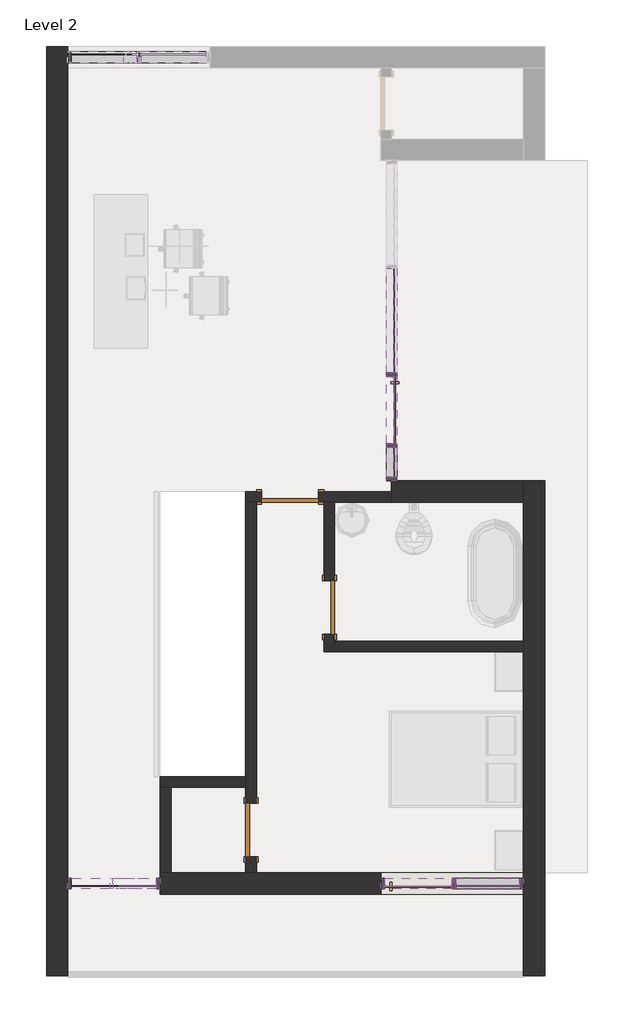
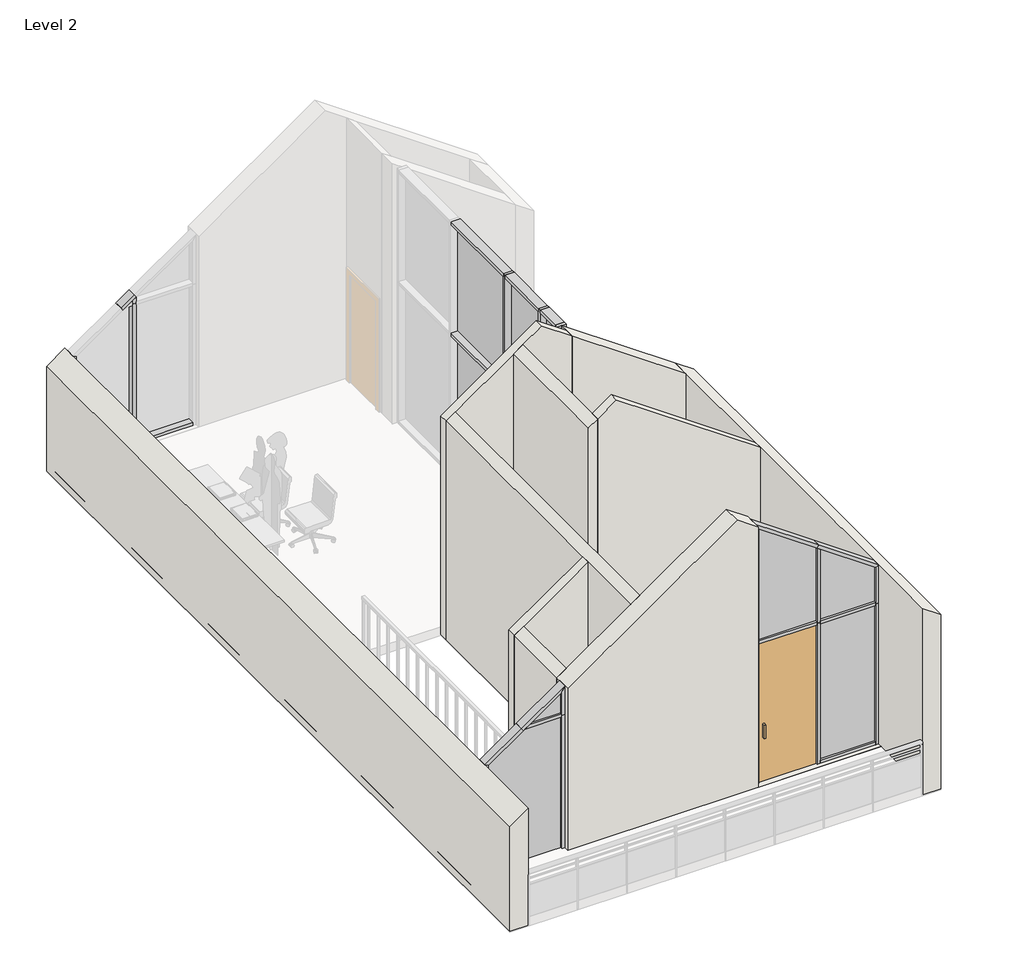
# One storey, part 1 of 2: 37 members, 10 plates, 10 walls, 5 doors.
"""IFC4 building model written with IfcOpenShell, lengths in millimetres."""

from ifc_helpers import new_model, si_unit, frame, origin, place, context, project, spatial, polyline, outline, extrude, faceted_brep, transform, mapped, element, save
from components import m_door_curtain_wall_single_glass_m_door_curtain_wall_single_b00c2793, m_door_curtain_wall_single_glass_m_door_curtain_wall_single_a386b0a2, m_door_single_flush_panel_double_acting_750_x_2000mm_e3d998e5, m_door_single_panel_750_x_2000mm_5cf0dcc2, m_door_single_panel_800_x_2100mm_d01656e8, rectangular_mullion_50_x_150mm_a91aaa2b, rectangular_mullion_50_x_150mm_6588f46c, rectangular_mullion_50_x_150mm_89c22e8d, rectangular_mullion_50_x_150mm_2615a836, rectangular_mullion_50_x_150mm_129a33a7, rectangular_mullion_50_x_150mm_c59a77fc, rectangular_mullion_50_x_150mm_4a18de0c, rectangular_mullion_50_x_150mm_a16d5dba, rectangular_mullion_50_x_150mm_59b4522d, rectangular_mullion_50_x_150mm_a5bab1e1, rectangular_mullion_50_x_150mm_e6be0bb7, rectangular_mullion_50_x_150mm_987ee5f5, rectangular_mullion_50_x_150mm_e09f09b0, rectangular_mullion_50_x_150mm_fd5e96fe, rectangular_mullion_50_x_150mm_9159db86, rectangular_mullion_50_x_150mm_405b5ff6, rectangular_mullion_50_x_150mm_a3343b62, rectangular_mullion_50_x_150mm_bd832bbd, rectangular_mullion_50_x_150mm_0164b494, rectangular_mullion_50_x_150mm_17c629a1, rectangular_mullion_50_x_150mm_35d6a770, rectangular_mullion_50_x_150mm_dd699d0b, rectangular_mullion_50_x_150mm_0e9b4e8c, rectangular_mullion_50_x_150mm_bef26404, rectangular_mullion_50_x_150mm_3ddb3363, rectangular_mullion_50_x_150mm_71cd5d06, rectangular_mullion_50_x_150mm_6afb4452, rectangular_mullion_50_x_150mm_b2f97b5b, system_panel_glazed_5205d833, system_panel_glazed_35c1503a, system_panel_glazed_def3cda3, system_panel_glazed_393e2e5d, system_panel_glazed_fc828323, system_panel_glazed_9e355314, system_panel_glazed_94ea2f12, system_panel_glazed_9142b3e3, system_panel_glazed_bc7b3e81, system_panel_glazed_03cdf4a0

model = new_model("IFC4")

# Units and contexts
model_context = context("Model", 3, world=origin())
ifc_project = project(units=[si_unit("LENGTHUNIT", "METRE", prefix="MILLI")], contexts=[model_context])

# Site, building, storey
site = spatial("IfcSite", under=ifc_project)
building = spatial("IfcBuilding", under=site)
storey = spatial("IfcBuildingStorey", under=building, Name="Level 2", Elevation=3200.0)

# Doors
placement = place(None, origin())
m_door_curtain_wall_single_glass_m_door_curtain_wall_single_shape = m_door_curtain_wall_single_glass_m_door_curtain_wall_single_b00c2793(model_context)
element("IfcDoor", 1, ObjectType="M_Door-Curtain-Wall-Single-Glass : M_Door-Curtain-Wall-Single-Glass", at=placement, inside=storey, context=model_context, shape_type="MappedRepresentation", body=[
    mapped(m_door_curtain_wall_single_glass_m_door_curtain_wall_single_shape, transform((-1444.0317552, -4266.7477501, 3333.3878119), x_axis=(1.0, 0.0, 0.0), y_axis=(0.0, 1.0, 0.0), z_axis=(0.0, 0.0, 1.0))),
])
m_door_curtain_wall_single_glass_m_door_curtain_wall_single_2_shape = m_door_curtain_wall_single_glass_m_door_curtain_wall_single_a386b0a2(model_context)
element("IfcDoor", 2, ObjectType="M_Door-Curtain-Wall-Single-Glass : M_Door-Curtain-Wall-Single-Glass", at=placement, inside=storey, context=model_context, shape_type="MappedRepresentation", body=[
    mapped(m_door_curtain_wall_single_glass_m_door_curtain_wall_single_2_shape, transform((-1819.0317552, 2379.0855833, 3340.0348366), x_axis=(0.0, -1.0, 0.0), y_axis=(1.0, 0.0, 0.0), z_axis=(0.0, 0.0, 1.0))),
])
m_door_single_flush_panel_double_acting_750_x_2000mm_shape = m_door_single_flush_panel_double_acting_750_x_2000mm_e3d998e5(model_context)
element("IfcDoor", 3, ObjectType="M_Door-Single-Flush_Panel_Double-Acting : 750 x 2000mm", at=placement, inside=storey, context=model_context, shape_type="MappedRepresentation", body=[
    mapped(m_door_single_flush_panel_double_acting_750_x_2000mm_shape, transform((-3794.0317552, -3516.7477501, 3200.0), x_axis=(0.0, 1.0, 0.0), y_axis=(-1.0, 0.0, 0.0), z_axis=(0.0, 0.0, 1.0))),
])
m_door_single_panel_750_x_2000mm_shape = m_door_single_panel_750_x_2000mm_5cf0dcc2(model_context)
element("IfcDoor", 4, ObjectType="M_Door-Single-Panel : 750 x 2000mm", at=placement, inside=storey, context=model_context, shape_type="MappedRepresentation", body=[
    mapped(m_door_single_panel_750_x_2000mm_shape, transform((-2694.0317552, -391.7477501, 3200.0), x_axis=(0.0, -1.0, 0.0), y_axis=(1.0, 0.0, 0.0), z_axis=(0.0, 0.0, 1.0))),
])
m_door_single_panel_800_x_2100mm_shape = m_door_single_panel_800_x_2100mm_d01656e8(model_context)
element("IfcDoor", 5, ObjectType="M_Door-Single-Panel : 800 x 2100mm", at=placement, inside=storey, context=model_context, shape_type="MappedRepresentation", body=[
    mapped(m_door_single_panel_800_x_2100mm_shape, transform((-3244.0317552, 1158.2522499, 3200.0), x_axis=(-1.0, 0.0, 0.0), y_axis=(0.0, -1.0, 0.0), z_axis=(0.0, 0.0, 1.0))),
])

# Members
rectangular_mullion_50_x_150mm_shape = rectangular_mullion_50_x_150mm_a91aaa2b(model_context)
element("IfcMember", 6, ObjectType="Rectangular Mullion : 50 x 150mm", at=placement, inside=storey, context=model_context, shape_type="MappedRepresentation", body=[
    mapped(rectangular_mullion_50_x_150mm_shape, transform((-6319.0317552, 7333.2522499, 3333.3878119), x_axis=(0.0, 0.0, -1.0), y_axis=(0.0, -1.0, 0.0), z_axis=(-1.0, 0.0, 0.0))),
])
element("IfcMember", 7, ObjectType="Rectangular Mullion : 50 x 150mm", at=placement, inside=storey, context=model_context, shape_type="MappedRepresentation", body=[
    mapped(rectangular_mullion_50_x_150mm_shape, transform((-5344.0317552, 7333.2522499, 3333.3878119), x_axis=(0.0, 0.0, -1.0), y_axis=(0.0, -1.0, 0.0), z_axis=(-1.0, 0.0, 0.0))),
])
rectangular_mullion_50_x_150mm_2_shape = rectangular_mullion_50_x_150mm_6588f46c(model_context)
element("IfcMember", 8, ObjectType="Rectangular Mullion : 50 x 150mm", at=placement, inside=storey, context=model_context, shape_type="MappedRepresentation", body=[
    mapped(rectangular_mullion_50_x_150mm_2_shape, transform((-5119.0317552, -4266.7477501, 3200.0), x_axis=(0.0, 0.0, -1.0), y_axis=(0.0, 1.0, 0.0), z_axis=(1.0, 0.0, 0.0))),
])
rectangular_mullion_50_x_150mm_3_shape = rectangular_mullion_50_x_150mm_89c22e8d(model_context)
element("IfcMember", 9, ObjectType="Rectangular Mullion : 50 x 150mm", at=placement, inside=storey, context=model_context, shape_type="MappedRepresentation", body=[
    mapped(rectangular_mullion_50_x_150mm_3_shape, transform((-1819.0317552, 1433.2522499, 7705.4462072), x_axis=(0.0, 0.0, 1.0), y_axis=(-1.0, 0.0, 0.0), z_axis=(0.0, -1.0, 0.0))),
])
rectangular_mullion_50_x_150mm_4_shape = rectangular_mullion_50_x_150mm_2615a836(model_context)
element("IfcMember", 10, ObjectType="Rectangular Mullion : 50 x 150mm", at=placement, inside=storey, context=model_context, shape_type="MappedRepresentation", body=[
    mapped(rectangular_mullion_50_x_150mm_4_shape, transform((-1919.0317552, -4266.7477501, 5758.3878119), x_axis=(0.0, 0.0, 1.0), y_axis=(0.0, 1.0, 0.0), z_axis=(-1.0, 0.0, 0.0))),
])
element("IfcMember", 11, ObjectType="Rectangular Mullion : 50 x 150mm", at=placement, inside=storey, context=model_context, shape_type="MappedRepresentation", body=[
    mapped(rectangular_mullion_50_x_150mm_3_shape, transform((-1819.0317552, 1858.2522499, 3340.0348366), x_axis=(0.0, 0.0, -1.0), y_axis=(-1.0, 0.0, 0.0), z_axis=(0.0, 1.0, 0.0))),
])
rectangular_mullion_50_x_150mm_5_shape = rectangular_mullion_50_x_150mm_129a33a7(model_context)
element("IfcMember", 12, ObjectType="Rectangular Mullion : 50 x 150mm", at=placement, inside=storey, context=model_context, shape_type="MappedRepresentation", body=[
    mapped(rectangular_mullion_50_x_150mm_5_shape, transform((-1819.0317552, 1433.2522499, 5765.0348366), x_axis=(0.0, 0.0, 1.0), y_axis=(-1.0, 0.0, 0.0), z_axis=(0.0, -1.0, 0.0))),
])
rectangular_mullion_50_x_150mm_6_shape = rectangular_mullion_50_x_150mm_c59a77fc(model_context)
element("IfcMember", 13, ObjectType="Rectangular Mullion : 50 x 150mm", at=placement, inside=storey, context=model_context, shape_type="MappedRepresentation", body=[
    mapped(rectangular_mullion_50_x_150mm_6_shape, transform((-5369.0317552, 7333.2522499, 3333.3878119), x_axis=(1.0, 0.0, 0.0), y_axis=(0.0, -1.0, 0.0), z_axis=(0.0, 0.0, -1.0))),
])
element("IfcMember", 14, ObjectType="Rectangular Mullion : 50 x 150mm", at=placement, inside=storey, context=model_context, shape_type="MappedRepresentation", body=[
    mapped(rectangular_mullion_50_x_150mm_6_shape, transform((-944.0317552, -4266.7477501, 3333.3878119), x_axis=(-1.0, 0.0, 0.0), y_axis=(0.0, 1.0, 0.0), z_axis=(0.0, 0.0, -1.0))),
])
element("IfcMember", 15, ObjectType="Rectangular Mullion : 50 x 150mm", at=placement, inside=storey, context=model_context, shape_type="MappedRepresentation", body=[
    mapped(rectangular_mullion_50_x_150mm_6_shape, transform((-1819.0317552, 2874.9189166, 3340.0348366), x_axis=(0.0, -1.0, 0.0), y_axis=(-1.0, 0.0, 0.0), z_axis=(0.0, 0.0, -1.0))),
])
element("IfcMember", 16, ObjectType="Rectangular Mullion : 50 x 150mm", at=placement, inside=storey, context=model_context, shape_type="MappedRepresentation", body=[
    mapped(rectangular_mullion_50_x_150mm_6_shape, transform((-1819.0317552, 1883.2522499, 3340.0348366), x_axis=(0.0, -1.0, 0.0), y_axis=(-1.0, 0.0, 0.0), z_axis=(0.0, 0.0, -1.0))),
])
rectangular_mullion_50_x_150mm_7_shape = rectangular_mullion_50_x_150mm_4a18de0c(model_context)
element("IfcMember", 17, ObjectType="Rectangular Mullion : 50 x 150mm", at=placement, inside=storey, context=model_context, shape_type="MappedRepresentation", body=[
    mapped(rectangular_mullion_50_x_150mm_7_shape, transform((-1819.0317552, 2899.9189166, 7705.4462072), x_axis=(0.0, 0.0, 1.0), y_axis=(-1.0, 0.0, 0.0), z_axis=(0.0, -1.0, 0.0))),
])
rectangular_mullion_50_x_150mm_8_shape = rectangular_mullion_50_x_150mm_a16d5dba(model_context)
element("IfcMember", 18, ObjectType="Rectangular Mullion : 50 x 150mm", at=placement, inside=storey, context=model_context, shape_type="MappedRepresentation", body=[
    mapped(rectangular_mullion_50_x_150mm_8_shape, transform((-1819.0317552, 2874.9189166, 5765.0348366), x_axis=(0.0, -1.0, 0.0), y_axis=(-1.0, 0.0, 0.0), z_axis=(0.0, 0.0, -1.0))),
])
element("IfcMember", 19, ObjectType="Rectangular Mullion : 50 x 150mm", at=placement, inside=storey, context=model_context, shape_type="MappedRepresentation", body=[
    mapped(rectangular_mullion_50_x_150mm_8_shape, transform((-1819.0317552, 1883.2522499, 5765.0348366), x_axis=(0.0, -1.0, 0.0), y_axis=(-1.0, 0.0, 0.0), z_axis=(0.0, 0.0, -1.0))),
])
rectangular_mullion_50_x_150mm_9_shape = rectangular_mullion_50_x_150mm_59b4522d(model_context)
element("IfcMember", 20, ObjectType="Rectangular Mullion : 50 x 150mm", at=placement, inside=storey, context=model_context, shape_type="MappedRepresentation", body=[
    mapped(rectangular_mullion_50_x_150mm_9_shape, transform((-1819.0317552, 2899.9189166, 5765.0348366), x_axis=(0.0, 0.0, 1.0), y_axis=(-1.0, 0.0, 0.0), z_axis=(0.0, -1.0, 0.0))),
])
rectangular_mullion_50_x_150mm_10_shape = rectangular_mullion_50_x_150mm_a5bab1e1(model_context)
element("IfcMember", 21, ObjectType="Rectangular Mullion : 50 x 150mm", at=placement, inside=storey, context=model_context, shape_type="MappedRepresentation", body=[
    mapped(rectangular_mullion_50_x_150mm_10_shape, transform((-1819.0317552, 1908.2522499, 5765.0348366), x_axis=(0.0, 0.0, 1.0), y_axis=(-1.0, 0.0, 0.0), z_axis=(0.0, -1.0, 0.0))),
])
rectangular_mullion_50_x_150mm_11_shape = rectangular_mullion_50_x_150mm_e6be0bb7(model_context)
element("IfcMember", 22, ObjectType="Rectangular Mullion : 50 x 150mm", at=placement, inside=storey, context=model_context, shape_type="MappedRepresentation", body=[
    mapped(rectangular_mullion_50_x_150mm_11_shape, transform((-1819.0317552, 1908.2522499, 7705.4462072), x_axis=(0.0, 0.0, 1.0), y_axis=(-1.0, 0.0, 0.0), z_axis=(0.0, -1.0, 0.0))),
])
rectangular_mullion_50_x_150mm_12_shape = rectangular_mullion_50_x_150mm_987ee5f5(model_context)
element("IfcMember", 23, ObjectType="Rectangular Mullion : 50 x 150mm", at=placement, inside=storey, context=model_context, shape_type="MappedRepresentation", body=[
    mapped(rectangular_mullion_50_x_150mm_12_shape, transform((-5369.0317552, 7333.2522499, 5910.2697997), x_axis=(-0.5735764363510469, 0.0, 0.8191520442889911), y_axis=(0.0, -1.0, 0.0), z_axis=(0.8191520442889911, 0.0, 0.5735764363510469))),
])
rectangular_mullion_50_x_150mm_13_shape = rectangular_mullion_50_x_150mm_e09f09b0(model_context)
element("IfcMember", 24, ObjectType="Rectangular Mullion : 50 x 150mm", at=placement, inside=storey, context=model_context, shape_type="MappedRepresentation", body=[
    mapped(rectangular_mullion_50_x_150mm_13_shape, transform((-5369.0317552, 7333.2522499, 5758.3878119), x_axis=(1.0, 0.0, 0.0), y_axis=(0.0, -1.0, 0.0), z_axis=(0.0, 0.0, -1.0))),
])
rectangular_mullion_50_x_150mm_14_shape = rectangular_mullion_50_x_150mm_fd5e96fe(model_context)
element("IfcMember", 25, ObjectType="Rectangular Mullion : 50 x 150mm", at=placement, inside=storey, context=model_context, shape_type="MappedRepresentation", body=[
    mapped(rectangular_mullion_50_x_150mm_14_shape, transform((-1819.0317552, 1383.2522499, 3340.0348366), x_axis=(0.0, -1.0, 0.0), y_axis=(-1.0, 0.0, 0.0), z_axis=(0.0, 0.0, -1.0))),
])
rectangular_mullion_50_x_150mm_15_shape = rectangular_mullion_50_x_150mm_9159db86(model_context)
element("IfcMember", 26, ObjectType="Rectangular Mullion : 50 x 150mm", at=placement, inside=storey, context=model_context, shape_type="MappedRepresentation", body=[
    mapped(rectangular_mullion_50_x_150mm_15_shape, transform((-6369.0317552, 7333.2522499, 5210.0622615), x_axis=(-1.0, 0.0, 0.0), y_axis=(0.0, -1.0, 0.0), z_axis=(0.0, 0.0, 1.0))),
])
rectangular_mullion_50_x_150mm_16_shape = rectangular_mullion_50_x_150mm_405b5ff6(model_context)
element("IfcMember", 27, ObjectType="Rectangular Mullion : 50 x 150mm", at=placement, inside=storey, context=model_context, shape_type="MappedRepresentation", body=[
    mapped(rectangular_mullion_50_x_150mm_16_shape, transform((-6369.0317552, -4266.7477501, 5210.0622615), x_axis=(-0.5735764363510464, 0.0, 0.8191520442889917), y_axis=(0.0, 1.0, 0.0), z_axis=(-0.8191520442889916, 0.0, -0.5735764363510463))),
])
rectangular_mullion_50_x_150mm_17_shape = rectangular_mullion_50_x_150mm_a3343b62(model_context)
element("IfcMember", 28, ObjectType="Rectangular Mullion : 50 x 150mm", at=placement, inside=storey, context=model_context, shape_type="MappedRepresentation", body=[
    mapped(rectangular_mullion_50_x_150mm_17_shape, transform((-5776.439251, -4266.7477501, 5625.0), x_axis=(-0.5735764363510472, 0.0, 0.8191520442889911), y_axis=(0.0, 1.0, 0.0), z_axis=(-0.819152044288991, 0.0, -0.573576436351047))),
])
rectangular_mullion_50_x_150mm_18_shape = rectangular_mullion_50_x_150mm_bd832bbd(model_context)
element("IfcMember", 29, ObjectType="Rectangular Mullion : 50 x 150mm", at=placement, inside=storey, context=model_context, shape_type="MappedRepresentation", body=[
    mapped(rectangular_mullion_50_x_150mm_18_shape, transform((-5776.439251, -4266.7477501, 5625.0), x_axis=(0.0, 0.0, 1.0), y_axis=(0.0, 1.0, 0.0), z_axis=(-1.0, 0.0, 0.0))),
])
rectangular_mullion_50_x_150mm_19_shape = rectangular_mullion_50_x_150mm_0164b494(model_context)
element("IfcMember", 30, ObjectType="Rectangular Mullion : 50 x 150mm", at=placement, inside=storey, context=model_context, shape_type="MappedRepresentation", body=[
    mapped(rectangular_mullion_50_x_150mm_19_shape, transform((-6369.0317552, -4266.7477501, 3200.0), x_axis=(-1.0, 0.0, 0.0), y_axis=(0.0, 1.0, 0.0), z_axis=(0.0, 0.0, -1.0))),
])
rectangular_mullion_50_x_150mm_20_shape = rectangular_mullion_50_x_150mm_17c629a1(model_context)
element("IfcMember", 31, ObjectType="Rectangular Mullion : 50 x 150mm", at=placement, inside=storey, context=model_context, shape_type="MappedRepresentation", body=[
    mapped(rectangular_mullion_50_x_150mm_20_shape, transform((-5069.0317552, -4266.7477501, 6120.3320611), x_axis=(1.0, 0.0, 0.0), y_axis=(0.0, 1.0, 0.0), z_axis=(0.0, 0.0, 1.0))),
])
rectangular_mullion_50_x_150mm_21_shape = rectangular_mullion_50_x_150mm_35d6a770(model_context)
element("IfcMember", 32, ObjectType="Rectangular Mullion : 50 x 150mm", at=placement, inside=storey, context=model_context, shape_type="MappedRepresentation", body=[
    mapped(rectangular_mullion_50_x_150mm_21_shape, transform((-19.0317552, -4266.7477501, 3333.3878119), x_axis=(0.0, 0.0, -1.0), y_axis=(0.0, 1.0, 0.0), z_axis=(1.0, 0.0, 0.0))),
])
rectangular_mullion_50_x_150mm_22_shape = rectangular_mullion_50_x_150mm_dd699d0b(model_context)
element("IfcMember", 33, ObjectType="Rectangular Mullion : 50 x 150mm", at=placement, inside=storey, context=model_context, shape_type="MappedRepresentation", body=[
    mapped(rectangular_mullion_50_x_150mm_22_shape, transform((-1969.0317552, -4266.7477501, 7810.4773379), x_axis=(0.5735764363510467, 0.0, 0.8191520442889915), y_axis=(0.0, 1.0, 0.0), z_axis=(-0.8191520442889915, 0.0, 0.5735764363510467))),
])
rectangular_mullion_50_x_150mm_23_shape = rectangular_mullion_50_x_150mm_0e9b4e8c(model_context)
element("IfcMember", 34, ObjectType="Rectangular Mullion : 50 x 150mm", at=placement, inside=storey, context=model_context, shape_type="MappedRepresentation", body=[
    mapped(rectangular_mullion_50_x_150mm_23_shape, transform((-944.0317552, -4266.7477501, 7092.7646112), x_axis=(0.5735764363510469, 0.0, 0.8191520442889912), y_axis=(0.0, 1.0, 0.0), z_axis=(-0.8191520442889912, 0.0, 0.5735764363510469))),
])
rectangular_mullion_50_x_150mm_24_shape = rectangular_mullion_50_x_150mm_bef26404(model_context)
element("IfcMember", 35, ObjectType="Rectangular Mullion : 50 x 150mm", at=placement, inside=storey, context=model_context, shape_type="MappedRepresentation", body=[
    mapped(rectangular_mullion_50_x_150mm_24_shape, transform((-944.0317552, -4266.7477501, 5758.3878119), x_axis=(-1.0, 0.0, 0.0), y_axis=(0.0, 1.0, 0.0), z_axis=(0.0, 0.0, -1.0))),
])
rectangular_mullion_50_x_150mm_25_shape = rectangular_mullion_50_x_150mm_3ddb3363(model_context)
element("IfcMember", 36, ObjectType="Rectangular Mullion : 50 x 150mm", at=placement, inside=storey, context=model_context, shape_type="MappedRepresentation", body=[
    mapped(rectangular_mullion_50_x_150mm_25_shape, transform((-919.0317552, -4266.7477501, 5758.3878119), x_axis=(0.0, 0.0, 1.0), y_axis=(0.0, 1.0, 0.0), z_axis=(-1.0, 0.0, 0.0))),
])
element("IfcMember", 37, ObjectType="Rectangular Mullion : 50 x 150mm", at=placement, inside=storey, context=model_context, shape_type="MappedRepresentation", body=[
    mapped(rectangular_mullion_50_x_150mm_14_shape, transform((-1969.0317552, -4266.7477501, 3333.3878119), x_axis=(-1.0, 0.0, 0.0), y_axis=(0.0, 1.0, 0.0), z_axis=(0.0, 0.0, -1.0))),
])
rectangular_mullion_50_x_150mm_26_shape = rectangular_mullion_50_x_150mm_71cd5d06(model_context)
element("IfcMember", 38, ObjectType="Rectangular Mullion : 50 x 150mm", at=placement, inside=storey, context=model_context, shape_type="MappedRepresentation", body=[
    mapped(rectangular_mullion_50_x_150mm_26_shape, transform((30.9682448, -4266.7477501, 6410.0622615), x_axis=(1.0, 0.0, 0.0), y_axis=(0.0, 1.0, 0.0), z_axis=(0.0, 0.0, 1.0))),
])
rectangular_mullion_50_x_150mm_27_shape = rectangular_mullion_50_x_150mm_6afb4452(model_context)
element("IfcMember", 39, ObjectType="Rectangular Mullion : 50 x 150mm", at=placement, inside=storey, context=model_context, shape_type="MappedRepresentation", body=[
    mapped(rectangular_mullion_50_x_150mm_27_shape, transform((-1819.0317552, 1383.2522499, 5765.0348366), x_axis=(0.0, -1.0, 0.0), y_axis=(-1.0, 0.0, 0.0), z_axis=(0.0, 0.0, -1.0))),
])
element("IfcMember", 40, ObjectType="Rectangular Mullion : 50 x 150mm", at=placement, inside=storey, context=model_context, shape_type="MappedRepresentation", body=[
    mapped(rectangular_mullion_50_x_150mm_14_shape, transform((-5069.0317552, -4266.7477501, 5625.0), x_axis=(1.0, 0.0, 0.0), y_axis=(0.0, 1.0, 0.0), z_axis=(0.0, 0.0, 1.0))),
])
element("IfcMember", 41, ObjectType="Rectangular Mullion : 50 x 150mm", at=placement, inside=storey, context=model_context, shape_type="MappedRepresentation", body=[
    mapped(rectangular_mullion_50_x_150mm_14_shape, transform((30.9682448, -4266.7477501, 5758.3878119), x_axis=(1.0, 0.0, 0.0), y_axis=(0.0, 1.0, 0.0), z_axis=(0.0, 0.0, 1.0))),
])
rectangular_mullion_50_x_150mm_28_shape = rectangular_mullion_50_x_150mm_b2f97b5b(model_context)
element("IfcMember", 42, ObjectType="Rectangular Mullion : 50 x 150mm", at=placement, inside=storey, context=model_context, shape_type="MappedRepresentation", body=[
    mapped(rectangular_mullion_50_x_150mm_28_shape, transform((-1969.0317552, -4266.7477501, 5758.3878119), x_axis=(-1.0, 0.0, 0.0), y_axis=(0.0, 1.0, 0.0), z_axis=(0.0, 0.0, -1.0))),
])

# Plates
system_panel_glazed_shape = system_panel_glazed_5205d833(model_context)
element("IfcPlate", 43, ObjectType="System Panel : Glazed", at=placement, inside=storey, context=model_context, shape_type="MappedRepresentation", body=[
    mapped(system_panel_glazed_shape, transform((-5719.0317552, -4266.7477501, 3250.0), x_axis=(-1.0, 0.0, 0.0), y_axis=(0.0, -1.0, 0.0), z_axis=(0.0, 0.0, 1.0))),
])
system_panel_glazed_2_shape = system_panel_glazed_35c1503a(model_context)
element("IfcPlate", 44, ObjectType="System Panel : Glazed", at=placement, inside=storey, context=model_context, shape_type="MappedRepresentation", body=[
    mapped(system_panel_glazed_2_shape, transform((-469.0317552, -4266.7477501, 3383.3878119), x_axis=(-1.0, 0.0, 0.0), y_axis=(0.0, -1.0, 0.0), z_axis=(0.0, 0.0, 1.0))),
])
system_panel_glazed_3_shape = system_panel_glazed_def3cda3(model_context)
element("IfcPlate", 45, ObjectType="System Panel : Glazed", at=placement, inside=storey, context=model_context, shape_type="MappedRepresentation", body=[
    mapped(system_panel_glazed_3_shape, transform((-1819.0317552, 3633.2522499, 3390.0348366), x_axis=(0.0, -1.0, 0.0), y_axis=(1.0, 0.0, 0.0), z_axis=(0.0, 0.0, 1.0))),
])
system_panel_glazed_4_shape = system_panel_glazed_393e2e5d(model_context)
element("IfcPlate", 46, ObjectType="System Panel : Glazed", at=placement, inside=storey, context=model_context, shape_type="MappedRepresentation", body=[
    mapped(system_panel_glazed_4_shape, transform((-1819.0317552, 3633.2522499, 5790.0348366), x_axis=(0.0, -1.0, 0.0), y_axis=(1.0, 0.0, 0.0), z_axis=(0.0, 0.0, 1.0))),
])
system_panel_glazed_5_shape = system_panel_glazed_fc828323(model_context)
element("IfcPlate", 47, ObjectType="System Panel : Glazed", at=placement, inside=storey, context=model_context, shape_type="MappedRepresentation", body=[
    mapped(system_panel_glazed_5_shape, transform((-1819.0317552, 2379.0855833, 5790.0348366), x_axis=(0.0, -1.0, 0.0), y_axis=(1.0, 0.0, 0.0), z_axis=(0.0, 0.0, 1.0))),
])
system_panel_glazed_6_shape = system_panel_glazed_9e355314(model_context)
element("IfcPlate", 48, ObjectType="System Panel : Glazed", at=placement, inside=storey, context=model_context, shape_type="MappedRepresentation", body=[
    mapped(system_panel_glazed_6_shape, transform((-5386.2974831, -4266.7477501, 5650.0), x_axis=(-1.0, 0.0, 0.0), y_axis=(0.0, -1.0, 0.0), z_axis=(0.0, 0.0, 1.0))),
])
system_panel_glazed_7_shape = system_panel_glazed_94ea2f12(model_context)
element("IfcPlate", 49, ObjectType="System Panel : Glazed", at=placement, inside=storey, context=model_context, shape_type="MappedRepresentation", body=[
    mapped(system_panel_glazed_7_shape, transform((-469.0317552, -4266.7477501, 5783.3878119), x_axis=(-1.0, 0.0, 0.0), y_axis=(0.0, -1.0, 0.0), z_axis=(0.0, 0.0, 1.0))),
])
system_panel_glazed_8_shape = system_panel_glazed_9142b3e3(model_context)
element("IfcPlate", 50, ObjectType="System Panel : Glazed", at=placement, inside=storey, context=model_context, shape_type="MappedRepresentation", body=[
    mapped(system_panel_glazed_8_shape, transform((-1444.0317552, -4266.7477501, 5783.3878119), x_axis=(-1.0, 0.0, 0.0), y_axis=(0.0, -1.0, 0.0), z_axis=(0.0, 0.0, 1.0))),
])
system_panel_glazed_9_shape = system_panel_glazed_bc7b3e81(model_context)
element("IfcPlate", 51, ObjectType="System Panel : Glazed", at=placement, inside=storey, context=model_context, shape_type="MappedRepresentation", body=[
    mapped(system_panel_glazed_9_shape, transform((-1819.0317552, 1645.7522499, 3390.0348366), x_axis=(0.0, -1.0, 0.0), y_axis=(1.0, 0.0, 0.0), z_axis=(0.0, 0.0, 1.0))),
])
system_panel_glazed_10_shape = system_panel_glazed_03cdf4a0(model_context)
element("IfcPlate", 52, ObjectType="System Panel : Glazed", at=placement, inside=storey, context=model_context, shape_type="MappedRepresentation", body=[
    mapped(system_panel_glazed_10_shape, transform((-1819.0317552, 1645.7522499, 5790.0348366), x_axis=(0.0, -1.0, 0.0), y_axis=(1.0, 0.0, 0.0), z_axis=(0.0, 0.0, 1.0))),
])

# Walls
element("IfcWall", 53, ObjectType="Generic - 300mm", at=placement, inside=storey, context=model_context, shape_type="Brep", body=[
    faceted_brep([(330.9682448, -5566.7477501, 3200.0), (330.9682448, 1383.2522499, 3200.0), (330.9682448, 1383.2522499, 6200.0), (330.9682448, -5566.7477501, 6200.0), (30.9682448, -5566.7477501, 3200.0), (30.9682448, -5566.7477501, 6410.0622615), (30.9682448, -1016.7477501, 6410.0622615), (30.9682448, -866.7477501, 6410.0622615), (30.9682448, 1083.2522499, 6410.0622615), (30.9682448, 1383.2522499, 6410.0622615), (30.9682448, 1383.2522499, 3200.0), (30.9682448, 1083.2522499, 3200.0), (30.9682448, -866.7477501, 3200.0), (30.9682448, -1016.7477501, 3200.0)], [[[0, 1, 2, 3]], [[4, 5, 6, 7, 8, 9, 10, 11, 12, 13]], [[1, 0, 4, 13, 12, 11, 10]], [[0, 3, 5, 4]], [[2, 1, 10, 9]], [[3, 2, 9, 8, 7, 6, 5]]]),
])
element("IfcWall", 54, ObjectType="Generic - 300mm", at=placement, inside=storey, context=model_context, shape_type="Brep", body=[
    faceted_brep([(-6669.0317552, 7483.2522499, 3200.0), (-6669.0317552, -5566.7477501, 3200.0), (-6669.0317552, -5566.7477501, 5000.0), (-6669.0317552, 7483.2522499, 5000.0), (-6369.0317552, 7483.2522499, 3200.0), (-6369.0317552, 7483.2522499, 5210.0622615), (-6369.0317552, -4116.7477501, 5210.0622615), (-6369.0317552, -4416.7477501, 5210.0622615), (-6369.0317552, -5566.7477501, 5210.0622615), (-6369.0317552, -5566.7477501, 3200.0), (-6369.0317552, -4416.7477501, 3200.0), (-6369.0317552, -4116.7477501, 3200.0)], [[[0, 1, 2, 3]], [[4, 5, 6, 7, 8, 9, 10, 11]], [[1, 0, 4, 11, 10, 9]], [[2, 1, 9, 8]], [[0, 3, 5, 4]], [[3, 2, 8, 7, 6, 5]]]),
])
element("IfcWall", 55, ObjectType="Generic - 300mm", at=placement, inside=storey, context=model_context, shape_type="Brep", body=[
    faceted_brep([(-1819.0317552, 1083.2522499, 3200.0), (30.9682448, 1083.2522499, 3200.0), (30.9682448, 1083.2522499, 6410.0622615), (-1819.0317552, 1083.2522499, 7705.4462072), (-1819.0317552, 1383.2522499, 3200.0), (-1819.0317552, 1383.2522499, 7705.4462072), (-1744.0317552, 1383.2522499, 7652.9306418), (30.9682448, 1383.2522499, 6410.0622615), (30.9682448, 1383.2522499, 3200.0), (-1819.0317552, 1233.2522499, 3200.0), (-1819.0317552, 1233.2522499, 7705.4462072)], [[[0, 1, 2, 3]], [[4, 5, 6, 7, 8]], [[1, 0, 9, 4, 8]], [[0, 3, 10, 5, 4, 9]], [[2, 1, 8, 7]], [[3, 2, 7, 6, 5, 10]]]),
])
element("IfcWall", 56, ObjectType="Generic - 300mm", at=placement, inside=storey, context=model_context, shape_type="Brep", body=[
    faceted_brep([(30.9682448, -4116.7477501, 3200.0), (-3719.0317552, -4116.7477501, 3200.0), (-3869.0317552, -4116.7477501, 3200.0), (-4919.0317552, -4116.7477501, 3200.0), (-5069.0317552, -4116.7477501, 3200.0), (-5069.0317552, -4116.7477501, 6120.3320611), (-4919.0317552, -4116.7477501, 6225.3631919), (-3869.0317552, -4116.7477501, 6960.581107), (-3719.0317552, -4116.7477501, 7065.6122377), (-2312.1429511, -4116.7477501, 8050.7263837), (-1969.0317552, -4116.7477501, 7810.4773379), (-1969.0317552, -4116.7477501, 3333.3878119), (30.9682448, -4116.7477501, 3333.3878119), (-5069.0317552, -4416.7477501, 3200.0), (30.9682448, -4416.7477501, 3200.0), (30.9682448, -4416.7477501, 3333.3878119), (-1969.0317552, -4416.7477501, 3333.3878119), (-1969.0317552, -4416.7477501, 7810.4773379), (-2312.1429511, -4416.7477501, 8050.7263837), (-5069.0317552, -4416.7477501, 6120.3320611)], [[[0, 1, 2, 3, 4, 5, 6, 7, 8, 9, 10, 11, 12]], [[13, 14, 15, 16, 17, 18, 19]], [[0, 14, 13, 4, 3, 2, 1]], [[14, 0, 12, 15]], [[5, 4, 13, 19]], [[16, 11, 10, 17]], [[11, 16, 15, 12]], [[9, 18, 17, 10]], [[18, 9, 8, 7, 6, 5, 19]]]),
])
element("IfcWall", 57, ObjectType="small inner wall 150mm", at=placement, inside=storey, context=model_context, shape_type="Brep", body=[
    faceted_brep([(-1819.0317552, 1233.2522499, 7705.4462072), (-1819.0317552, 1233.2522499, 3200.0), (-2844.0317552, 1233.2522499, 3200.0), (-2844.0317552, 1233.2522499, 5300.0), (-3644.0317552, 1233.2522499, 5300.0), (-3644.0317552, 1233.2522499, 3200.0), (-3869.0317552, 1233.2522499, 3200.0), (-3869.0317552, 1233.2522499, 6960.581107), (-2312.1429511, 1233.2522499, 8050.7263837), (-1819.0317552, 1083.2522499, 3200.0), (-1819.0317552, 1083.2522499, 7705.4462072), (-2312.1429511, 1083.2522499, 8050.7263837), (-2619.0317552, 1083.2522499, 7835.8405297), (-2769.0317552, 1083.2522499, 7730.809399), (-3719.0317552, 1083.2522499, 7065.6122377), (-3869.0317552, 1083.2522499, 6960.581107), (-3869.0317552, 1083.2522499, 3200.0), (-3719.0317552, 1083.2522499, 3200.0), (-3644.0317552, 1083.2522499, 3200.0), (-3644.0317552, 1083.2522499, 5300.0), (-2844.0317552, 1083.2522499, 5300.0), (-2844.0317552, 1083.2522499, 3200.0), (-2769.0317552, 1083.2522499, 3200.0), (-2619.0317552, 1083.2522499, 3200.0)], [[[0, 1, 2, 3, 4, 5, 6, 7, 8]], [[9, 10, 11, 12, 13, 14, 15, 16, 17, 18, 19, 20, 21, 22, 23]], [[16, 6, 5, 18, 17]], [[1, 9, 23, 22, 21, 2]], [[1, 0, 10, 9]], [[7, 6, 16, 15]], [[4, 19, 18, 5]], [[20, 3, 2, 21]], [[10, 0, 8, 11]], [[7, 15, 14, 13, 12, 11, 8]], [[3, 20, 19, 4]]]),
])
element("IfcWall", 58, ObjectType="small inner wall 150mm", at=placement, inside=storey, context=model_context, shape_type="Brep", body=[
    faceted_brep([(-3869.0317552, 1083.2522499, 6960.581107), (-3869.0317552, 1083.2522499, 3200.0), (-3869.0317552, -2766.7477501, 3200.0), (-3869.0317552, -2916.7477501, 3200.0), (-3869.0317552, -3141.7477501, 3200.0), (-3869.0317552, -3141.7477501, 5200.0), (-3869.0317552, -3891.7477501, 5200.0), (-3869.0317552, -3891.7477501, 3200.0), (-3869.0317552, -4116.7477501, 3200.0), (-3869.0317552, -4116.7477501, 6960.581107), (-3869.0317552, -2916.7477501, 6960.581107), (-3869.0317552, -2766.7477501, 6960.581107), (-3719.0317552, 1083.2522499, 3200.0), (-3719.0317552, 1083.2522499, 7065.6122377), (-3719.0317552, -4116.7477501, 7065.6122377), (-3719.0317552, -4116.7477501, 3200.0), (-3719.0317552, -3891.7477501, 3200.0), (-3719.0317552, -3891.7477501, 5200.0), (-3719.0317552, -3141.7477501, 5200.0), (-3719.0317552, -3141.7477501, 3200.0)], [[[0, 1, 2, 3, 4, 5, 6, 7, 8, 9, 10, 11]], [[12, 13, 14, 15, 16, 17, 18, 19]], [[1, 12, 19, 4, 3, 2]], [[15, 8, 7, 16]], [[1, 0, 13, 12]], [[9, 8, 15, 14]], [[18, 5, 4, 19]], [[6, 17, 16, 7]], [[0, 11, 10, 9, 14, 13]], [[17, 6, 5, 18]]]),
])
element("IfcWall", 59, ObjectType="small inner wall 150mm", at=placement, inside=storey, context=model_context, shape_type="Brep", body=[
    faceted_brep([(-3869.0317552, -2766.7477501, 3200.0), (-5069.0317552, -2766.7477501, 3200.0), (-5069.0317552, -2766.7477501, 6120.3320611), (-3869.0317552, -2766.7477501, 6960.581107), (-3869.0317552, -2916.7477501, 3200.0), (-3869.0317552, -2916.7477501, 6960.581107), (-4919.0317552, -2916.7477501, 6225.3631919), (-5069.0317552, -2916.7477501, 6120.3320611), (-5069.0317552, -2916.7477501, 3200.0), (-4919.0317552, -2916.7477501, 3200.0)], [[[0, 1, 2, 3]], [[4, 5, 6, 7, 8, 9]], [[1, 0, 4, 9, 8]], [[2, 1, 8, 7]], [[0, 3, 5, 4]], [[3, 2, 7, 6, 5]]]),
])
element("IfcWall", 60, ObjectType="small inner wall 150mm", at=placement, inside=storey, context=model_context, shape_type="SweptSolid", body=[
    extrude(outline(polyline([(6120.3320611, -5069.0317552), (3200.0, -5069.0317552), (3200.0, -4919.0317552), (6225.3631919, -4919.0317552), (6120.3320611, -5069.0317552)])), frame((0.0, -4116.7477501, 0.0), z_axis=(0.0, 1.0, 0.0), x_axis=(0.0, 0.0, 1.0)), (0.0, 0.0, 1.0), 1200.0),
])
element("IfcWall", 61, ObjectType="small inner wall 150mm", at=placement, inside=storey, context=model_context, shape_type="Brep", body=[
    faceted_brep([(-2769.0317552, 1083.2522499, 7730.809399), (-2769.0317552, 1083.2522499, 3200.0), (-2769.0317552, -16.7477501, 3200.0), (-2769.0317552, -16.7477501, 5200.0), (-2769.0317552, -766.7477501, 5200.0), (-2769.0317552, -766.7477501, 3200.0), (-2769.0317552, -1016.7477501, 3200.0), (-2769.0317552, -1016.7477501, 7730.809399), (-2619.0317552, 1083.2522499, 3200.0), (-2619.0317552, 1083.2522499, 7835.8405297), (-2619.0317552, -866.7477501, 7835.8405297), (-2619.0317552, -1016.7477501, 7835.8405297), (-2619.0317552, -1016.7477501, 3200.0), (-2619.0317552, -866.7477501, 3200.0), (-2619.0317552, -766.7477501, 3200.0), (-2619.0317552, -766.7477501, 5200.0), (-2619.0317552, -16.7477501, 5200.0), (-2619.0317552, -16.7477501, 3200.0)], [[[0, 1, 2, 3, 4, 5, 6, 7]], [[8, 9, 10, 11, 12, 13, 14, 15, 16, 17]], [[1, 8, 17, 2]], [[12, 6, 5, 14, 13]], [[1, 0, 9, 8]], [[7, 6, 12, 11]], [[4, 15, 14, 5]], [[16, 3, 2, 17]], [[0, 7, 11, 10, 9]], [[3, 16, 15, 4]]]),
])
element("IfcWall", 62, ObjectType="small inner wall 150mm", at=placement, inside=storey, context=model_context, shape_type="SweptSolid", body=[
    extrude(outline(polyline([(3200.0, -2619.0317552), (3200.0, 30.9682448), (6410.0622615, 30.9682448), (8050.7263837, -2312.1429511), (7835.8405297, -2619.0317552), (3200.0, -2619.0317552)])), frame((0.0, -1016.7477501, 0.0), z_axis=(0.0, 1.0, 0.0), x_axis=(0.0, 0.0, 1.0)), (0.0, 0.0, 1.0), 150.0),
])

save(model, "model.ifc")

# Revit data of these elements
# Type "M_Door-Curtain-Wall-Single-Glass : M_Door-Curtain-Wall-Single-Glass"
#   Type Mark = "46"
#   Assembly Code = "B2030100"
#   Analytic Construction = "<None>"
#   Width [instance default] = 900 mm
#   Thermal Resistance (R) = 1.7611 (m²·K)/W
#   Swing Angle [instance default] = 90.00°
#   Heat Transfer Coefficient (U) = 0.567826 W/(m²·K)
#   Offset = 50.8 mm
#   Define Thermal Properties by = 1
#   Function = 1
#   Door Handle Material = Aluminum
#   Glazing = Glass
#   Visual Light Transmittance = 0
#   Solar Heat Gain Coefficient = 0
#   Construction Type Id = ""
# Type "M_Door-Single-Flush_Panel_Double-Acting : 750 x 2000mm"
#   Type Mark = "45"
#   Construction Type Id = "DOOR"
#   Assembly Code = "C1020300"
#   Analytic Construction = "Wooden"
#   Thickness = 50 mm
#   Thermal Resistance (R) = 0.455703 (m²·K)/W
#   Swing Angle [instance default] = 90.00°
#   Heat Transfer Coefficient (U) = 2.19465 W/(m²·K)
#   Height = 2000 mm
#   Trim Projection Ext. = 25 mm
#   Trim Projection Int. = 25 mm
#   Trim Width Ext. = 80 mm
#   Trim Width Int. = 80 mm
#   Width = 750 mm
#   Define Thermal Properties by = 1
#   Trim Material = Paint - Sienna
#   Panel Material = Wood - Birch - Solid Stained Light Low Gloss
#   Visual Light Transmittance = 0
#   Solar Heat Gain Coefficient = 0
#   Function = (empty or 0)
#   Wall Closure = (empty or 0)
# Type "M_Door-Single-Panel : 750 x 2000mm"
#   Type Mark = "42"
#   Construction Type Id = "DOOR"
#   Assembly Code = "C1020300"
#   Analytic Construction = "Wooden"
#   Thickness = 50 mm
#   Thermal Resistance (R) = 0.455703 (m²·K)/W
#   Swing Angle [instance default] = 90.00°
#   Heat Transfer Coefficient (U) = 2.19465 W/(m²·K)
#   Height = 2000 mm
#   Trim Projection Ext = 25 mm
#   Trim Projection Int = 25 mm
#   Trim Width = 80 mm
#   Width = 750 mm
#   Define Thermal Properties by = 1
#   Panel Material = Wood - Birch - Solid Stained Light Low Gloss
#   Trim Material = Paint - Sienna
#   Visual Light Transmittance = 0
#   Solar Heat Gain Coefficient = 0
#   Function = (empty or 0)
#   Wall Closure = (empty or 0)
# Type "M_Door-Single-Panel : 800 x 2100mm"
#   Type Mark = "41"
#   Construction Type Id = "DOOR"
#   Assembly Code = "C1020300"
#   Analytic Construction = "Wooden"
#   Thickness = 50 mm
#   Thermal Resistance (R) = 0.455703 (m²·K)/W
#   Swing Angle [instance default] = 90.00°
#   Heat Transfer Coefficient (U) = 2.19465 W/(m²·K)
#   Height = 2100 mm
#   Trim Projection Ext = 25 mm
#   Trim Projection Int = 25 mm
#   Trim Width = 80 mm
#   Width = 800 mm
#   Define Thermal Properties by = 1
#   Panel Material = Wood - Birch - Solid Stained Light Low Gloss
#   Trim Material = Paint - Sienna
#   Visual Light Transmittance = 0
#   Solar Heat Gain Coefficient = 0
#   Function = (empty or 0)
#   Wall Closure = (empty or 0)
# Type "Rectangular Mullion : 50 x 150mm"
#   built-in parameter 1007304 = 0.492126 (stored number, unit not read)
#   built-in parameter 1007301 = 0.082021 (stored number, unit not read)
#   built-in parameter 1007300 = 0.082021 (stored number, unit not read)
# Type "System Panel : Glazed"
#   Construction Type Id = "GSP4R"
#   Analytic Construction = "1/8 in Pilkington single glazing"
#   Visual Light Transmittance = 0.9
#   Solar Heat Gain Coefficient = 0.86
#   Heat Transfer Coefficient (U) = 6.7069 W/(m²·K)
#   Define Thermal Properties by = 1
# Type "Generic - 300mm"
#   Layers, outside or top first: 300 mm no material (function 1)
# Type "small inner wall 150mm"
#   Layers, outside or top first: 150 mm no material (function 1)
# Elements 1, 2 (IfcDoor, "M_Door-Curtain-Wall-Single-Glass : M_Door-Curtain-Wall-Single-Glass")
#   Phase Created = New Construction
#   Materials on its faces: "Aluminum", "Glass"
# Element 3 (IfcDoor, "M_Door-Single-Flush_Panel_Double-Acting : 750 x 2000mm")
#   Swing Angle = 90.00°
#   Phase Created = New Construction
#   Materials on its faces: "Paint - Sienna", "Wood - Birch - Solid Stained Light Low Gloss"
# Element 4 (IfcDoor, "M_Door-Single-Panel : 750 x 2000mm")
#   Swing Angle = 90.00°
#   Phase Created = New Construction
#   Materials on its faces: "Paint - Sienna", "Wood - Birch - Solid Stained Light Low Gloss"
# Element 5 (IfcDoor, "M_Door-Single-Panel : 800 x 2100mm")
#   Swing Angle = 90.00°
#   Phase Created = New Construction
#   Materials on its faces: "Paint - Sienna", "Wood - Birch - Solid Stained Light Low Gloss"
# Elements 6, 7, 8, 9, 10, 11, 12, 13, 14, 15, 16, 17, 18, 19, 20, 21, 22, 23, 24, 25, 26, 27, 28, 29, 30, 31, 32, 33, 34, 35, 36, 37, 38, 39, 40, 41, 42 (IfcMember, "Rectangular Mullion : 50 x 150mm")
#   Phase Created = New Construction
#   Materials on its faces: "Aluminium"
# Elements 43, 44, 45, 46, 47, 48, 49, 50, 51, 52 (IfcPlate, "System Panel : Glazed")
#   Phase Created = New Construction
#   Materials on its faces: "Default New Material(6)"
# Element 53 (IfcWall, "Generic - 300mm")
#   Top Offset = 0 mm
#   Base Offset = 0 mm
#   wall height = 1800 mm
#   Phase Created = New Construction
#   Base Constraint = Level 2
#   Top Constraint = Level 3
#   Materials on its faces: "Default New Material(9)", "Default Wall", "Paint - Sienna"
# Element 54 (IfcWall, "Generic - 300mm")
#   Top Offset = 0 mm
#   Base Offset = 0 mm
#   wall height = 1800 mm
#   Phase Created = New Construction
#   Base Constraint = Level 2
#   Top Constraint = Level 3
#   Materials on its faces: "Default New Material(9)", "Default Wall", "Textile - Slate Blue"
# Element 55 (IfcWall, "Generic - 300mm")
#   Top Offset = 0 mm
#   Base Offset = 0 mm
#   wall height = 1800 mm
#   Phase Created = New Construction
#   Base Constraint = Level 2
#   Top Constraint = Level 3
#   Materials on its faces: "Default Wall", "Paint - Sienna", "Default New Material(9)"
# Element 56 (IfcWall, "Generic - 300mm")
#   Top Offset = 0 mm
#   Base Offset = 0 mm
#   wall height = 1800 mm
#   Phase Created = New Construction
#   Base Constraint = Level 2
#   Top Constraint = Level 3
#   Materials on its faces: "Default Wall", "Default New Material(9)"
# Element 57 (IfcWall, "small inner wall 150mm")
#   Top Offset = 0 mm
#   Base Offset = 0 mm
#   wall height = 1800 mm
#   Phase Created = New Construction
#   Base Constraint = Level 2
#   Top Constraint = Level 3
#   Materials on its faces: "Default Wall", "Textile - Slate Blue", "Paint - Sienna"
# Elements 58, 59, 60 (IfcWall, "small inner wall 150mm")
#   Top Offset = 0 mm
#   Base Offset = 0 mm
#   wall height = 1800 mm
#   Phase Created = New Construction
#   Base Constraint = Level 2
#   Top Constraint = Level 3
#   Materials on its faces: "Default Wall", "Textile - Slate Blue"
# Elements 61, 62 (IfcWall, "small inner wall 150mm")
#   Top Offset = 0 mm
#   Base Offset = 0 mm
#   wall height = 1800 mm
#   Phase Created = New Construction
#   Base Constraint = Level 2
#   Top Constraint = Level 3
#   Materials on its faces: "Default Wall", "Paint - Sienna"
# Materials
#   "Aluminum": class "Metal", colour RGB 247 247 247, transparency 0, Description = "Aluminum 6061", Cost = 0
#   "Glass": class "Glass", colour RGB 0 128 192, transparency 0.9, Description = "Soda Lime Glass", Cost = 0
#   "Paint - Sienna": colour RGB 118 70 51, transparency 0, Cost = 0
#   "Wood - Birch - Solid Stained Light Low Gloss": class "Wood", colour RGB 210 159 95, transparency 0, Cost = 0
#   "Aluminium": class "Metal", colour RGB 247 247 247, transparency 0, Description = "Aluminium 6061", Cost = 0
#   "Default New Material(6)": class "Generic", colour RGB 191 25 25, transparency 0.9, Cost = 0
#   "Default New Material(9)": class "Generic", colour RGB 63 63 64, transparency 0, Cost = 0
#   "Default Wall": colour RGB 128 128 128, transparency 0, Cost = 0
#   "Textile - Slate Blue": class "Fabric", colour RGB 98 102 118, transparency 0
